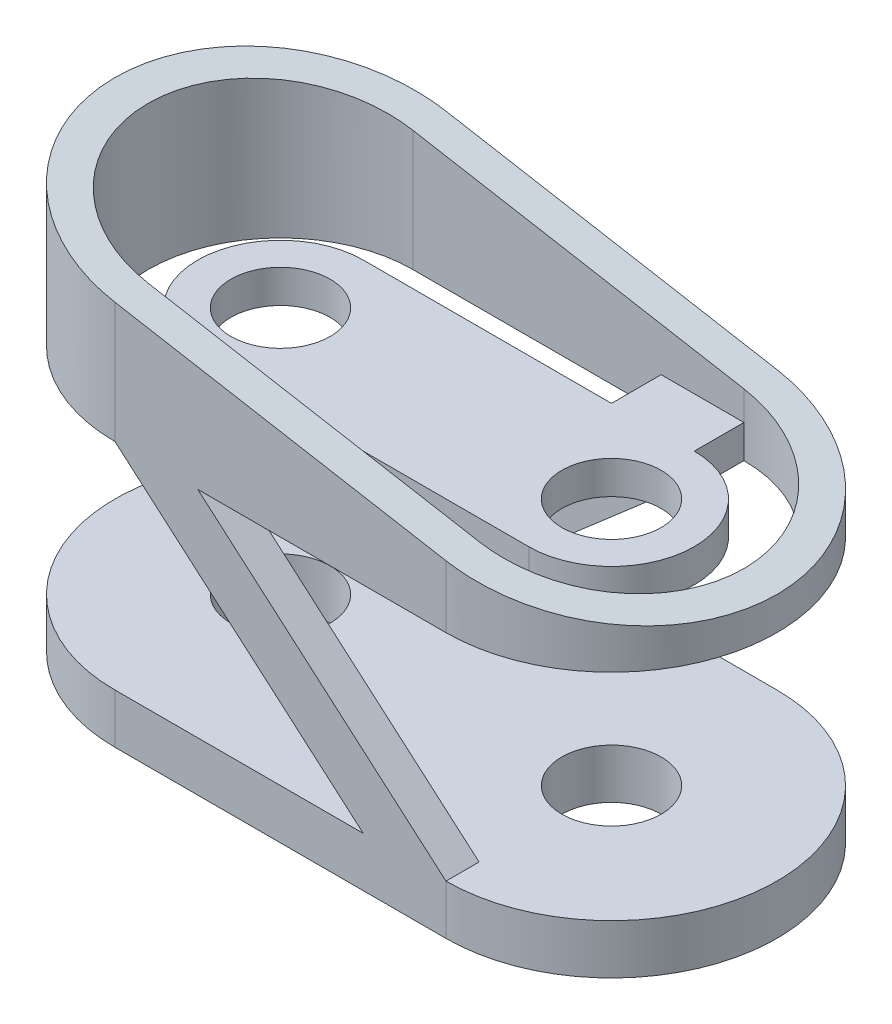
ISO-10303-21;
HEADER;
FILE_DESCRIPTION(('STEP AP214'),'2;1');
FILE_NAME('part.step','',(''),(''),'','','');
FILE_SCHEMA(('AUTOMOTIVE_DESIGN { 1 0 10303 214 1 1 1 1 }'));
ENDSEC;
DATA;
#1=APPLICATION_CONTEXT('core data for automotive mechanical design processes');
#2=APPLICATION_PROTOCOL_DEFINITION('international standard','automotive_design',2000,#1);
#3=PRODUCT_CONTEXT('',#1,'mechanical');
#4=PRODUCT('Part','Part','',(#3));
#5=PRODUCT_RELATED_PRODUCT_CATEGORY('part','',(#4));
#6=PRODUCT_DEFINITION_FORMATION('','',#4);
#7=PRODUCT_DEFINITION_CONTEXT('part definition',#1,'design');
#8=PRODUCT_DEFINITION('design','',#6,#7);
#9=PRODUCT_DEFINITION_SHAPE('','',#8);
#10=(LENGTH_UNIT() NAMED_UNIT(*) SI_UNIT(.MILLI.,.METRE.));
#11=(NAMED_UNIT(*) PLANE_ANGLE_UNIT() SI_UNIT($,.RADIAN.));
#12=(NAMED_UNIT(*) SI_UNIT($,.STERADIAN.) SOLID_ANGLE_UNIT());
#13=UNCERTAINTY_MEASURE_WITH_UNIT(LENGTH_MEASURE(1.E-05),#10,'distance_accuracy_value','');
#14=(GEOMETRIC_REPRESENTATION_CONTEXT(3) GLOBAL_UNCERTAINTY_ASSIGNED_CONTEXT((#13)) GLOBAL_UNIT_ASSIGNED_CONTEXT((#10,
#11,#12)) REPRESENTATION_CONTEXT('',''));
#15=CARTESIAN_POINT('',(0.,0.,0.));
#16=DIRECTION('',(0.,0.,1.));
#17=DIRECTION('',(1.,0.,0.));
#18=AXIS2_PLACEMENT_3D('',#15,#16,#17);
#19=CARTESIAN_POINT('',(0.,80.,0.));
#20=DIRECTION('',(0.,1.,0.));
#21=DIRECTION('',(0.,0.,1.));
#22=AXIS2_PLACEMENT_3D('',#19,#20,#21);
#23=PLANE('',#22);
#24=DIRECTION('',(-1.,0.,0.));
#25=VECTOR('',#24,1.);
#26=CARTESIAN_POINT('',(100.,80.,-50.));
#27=LINE('',#26,#25);
#28=CARTESIAN_POINT('',(75.,80.,-50.));
#29=VERTEX_POINT('',#28);
#30=CARTESIAN_POINT('',(0.,80.,-50.));
#31=VERTEX_POINT('',#30);
#32=EDGE_CURVE('E364',#29,#31,#27,.T.);
#33=ORIENTED_EDGE('',*,*,#32,.F.);
#34=DIRECTION('',(0.,0.,-1.));
#35=VECTOR('',#34,1.);
#36=CARTESIAN_POINT('',(75.,80.,-40.));
#37=LINE('',#36,#35);
#38=CARTESIAN_POINT('',(75.,80.,-40.));
#39=VERTEX_POINT('',#38);
#40=EDGE_CURVE('E470',#39,#29,#37,.T.);
#41=ORIENTED_EDGE('',*,*,#40,.F.);
#42=DIRECTION('',(-1.,0.,0.));
#43=VECTOR('',#42,1.);
#44=CARTESIAN_POINT('',(0.,80.,-40.));
#45=LINE('',#44,#43);
#46=CARTESIAN_POINT('',(0.,80.,-40.));
#47=VERTEX_POINT('',#46);
#48=EDGE_CURVE('E264',#39,#47,#45,.T.);
#49=ORIENTED_EDGE('',*,*,#48,.T.);
#50=CARTESIAN_POINT('',(0.,80.,0.));
#51=DIRECTION('',(0.,1.,0.));
#52=DIRECTION('',(0.,0.,1.));
#53=AXIS2_PLACEMENT_3D('',#50,#51,#52);
#54=CIRCLE('',#53,40.);
#55=CARTESIAN_POINT('',(0.,80.,40.));
#56=VERTEX_POINT('',#55);
#57=EDGE_CURVE('E345',#47,#56,#54,.T.);
#58=ORIENTED_EDGE('',*,*,#57,.T.);
#59=DIRECTION('',(0.,0.,1.));
#60=VECTOR('',#59,1.);
#61=CARTESIAN_POINT('',(0.,80.,40.));
#62=LINE('',#61,#60);
#63=CARTESIAN_POINT('',(0.,80.,50.));
#64=VERTEX_POINT('',#63);
#65=EDGE_CURVE('E393',#56,#64,#62,.T.);
#66=ORIENTED_EDGE('',*,*,#65,.T.);
#67=CARTESIAN_POINT('',(0.,80.,0.));
#68=DIRECTION('',(0.,1.,0.));
#69=DIRECTION('',(0.,0.,1.));
#70=AXIS2_PLACEMENT_3D('',#67,#68,#69);
#71=CIRCLE('',#70,50.);
#72=EDGE_CURVE('E358',#31,#64,#71,.T.);
#73=ORIENTED_EDGE('',*,*,#72,.F.);
#74=EDGE_LOOP('',(#33,#41,#49,#58,#66,#73));
#75=FACE_BOUND('',#74,.T.);
#76=ADVANCED_FACE('F43',(#75),#23,.F.);
#77=CARTESIAN_POINT('',(100.,80.,0.));
#78=DIRECTION('',(0.,1.,0.));
#79=DIRECTION('',(0.,0.,1.));
#80=AXIS2_PLACEMENT_3D('',#77,#78,#79);
#81=CIRCLE('',#80,40.);
#82=CARTESIAN_POINT('',(100.,80.,40.));
#83=VERTEX_POINT('',#82);
#84=CARTESIAN_POINT('',(100.,80.,-40.));
#85=VERTEX_POINT('',#84);
#86=EDGE_CURVE('E252',#83,#85,#81,.T.);
#87=ORIENTED_EDGE('',*,*,#86,.T.);
#88=DIRECTION('',(0.,0.,-1.));
#89=VECTOR('',#88,1.);
#90=CARTESIAN_POINT('',(100.,80.,-40.));
#91=LINE('',#90,#89);
#92=CARTESIAN_POINT('',(100.,80.,-50.));
#93=VERTEX_POINT('',#92);
#94=EDGE_CURVE('E209',#85,#93,#91,.T.);
#95=ORIENTED_EDGE('',*,*,#94,.T.);
#96=CARTESIAN_POINT('',(100.,80.,0.));
#97=DIRECTION('',(0.,1.,0.));
#98=DIRECTION('',(0.,0.,1.));
#99=AXIS2_PLACEMENT_3D('',#96,#97,#98);
#100=CIRCLE('',#99,50.);
#101=CARTESIAN_POINT('',(100.,80.,50.));
#102=VERTEX_POINT('',#101);
#103=EDGE_CURVE('E363',#102,#93,#100,.T.);
#104=ORIENTED_EDGE('',*,*,#103,.F.);
#105=DIRECTION('',(1.,0.,0.));
#106=VECTOR('',#105,1.);
#107=CARTESIAN_POINT('',(0.,80.,50.));
#108=LINE('',#107,#106);
#109=CARTESIAN_POINT('',(25.,80.,50.));
#110=VERTEX_POINT('',#109);
#111=EDGE_CURVE('E360',#110,#102,#108,.T.);
#112=ORIENTED_EDGE('',*,*,#111,.F.);
#113=DIRECTION('',(0.,0.,1.));
#114=VECTOR('',#113,1.);
#115=CARTESIAN_POINT('',(25.,80.,40.));
#116=LINE('',#115,#114);
#117=CARTESIAN_POINT('',(25.,80.,40.));
#118=VERTEX_POINT('',#117);
#119=EDGE_CURVE('E399',#118,#110,#116,.T.);
#120=ORIENTED_EDGE('',*,*,#119,.F.);
#121=DIRECTION('',(1.,0.,0.));
#122=VECTOR('',#121,1.);
#123=CARTESIAN_POINT('',(0.,80.,40.));
#124=LINE('',#123,#122);
#125=EDGE_CURVE('E263',#118,#83,#124,.T.);
#126=ORIENTED_EDGE('',*,*,#125,.T.);
#127=EDGE_LOOP('',(#87,#95,#104,#112,#120,#126));
#128=FACE_BOUND('',#127,.T.);
#129=ADVANCED_FACE('F258',(#128),#23,.F.);
#130=CARTESIAN_POINT('',(0.,15.,0.));
#131=DIRECTION('',(0.,-1.,0.));
#132=DIRECTION('',(0.,0.,-1.));
#133=AXIS2_PLACEMENT_3D('',#130,#131,#132);
#134=CYLINDRICAL_SURFACE('',#133,50.);
#135=CARTESIAN_POINT('',(0.,0.,0.));
#136=DIRECTION('',(0.,1.,0.));
#137=DIRECTION('',(0.,0.,1.));
#138=AXIS2_PLACEMENT_3D('',#135,#136,#137);
#139=CIRCLE('',#138,50.);
#140=CARTESIAN_POINT('',(0.,0.,-50.));
#141=VERTEX_POINT('',#140);
#142=CARTESIAN_POINT('',(0.,0.,50.));
#143=VERTEX_POINT('',#142);
#144=EDGE_CURVE('E411',#141,#143,#139,.T.);
#145=ORIENTED_EDGE('',*,*,#144,.T.);
#146=DIRECTION('',(0.,-1.,0.));
#147=VECTOR('',#146,1.);
#148=CARTESIAN_POINT('',(0.,15.,50.));
#149=LINE('',#148,#147);
#150=CARTESIAN_POINT('',(0.,15.,50.));
#151=VERTEX_POINT('',#150);
#152=EDGE_CURVE('E11',#151,#143,#149,.T.);
#153=ORIENTED_EDGE('',*,*,#152,.F.);
#154=CARTESIAN_POINT('',(0.,15.,0.));
#155=DIRECTION('',(0.,1.,0.));
#156=DIRECTION('',(0.,0.,1.));
#157=AXIS2_PLACEMENT_3D('',#154,#155,#156);
#158=CIRCLE('',#157,50.);
#159=CARTESIAN_POINT('',(0.,15.,-50.));
#160=VERTEX_POINT('',#159);
#161=EDGE_CURVE('E420',#160,#151,#158,.T.);
#162=ORIENTED_EDGE('',*,*,#161,.F.);
#163=DIRECTION('',(0.,-1.,0.));
#164=VECTOR('',#163,1.);
#165=CARTESIAN_POINT('',(0.,15.,-50.));
#166=LINE('',#165,#164);
#167=EDGE_CURVE('E431',#160,#141,#166,.T.);
#168=ORIENTED_EDGE('',*,*,#167,.T.);
#169=EDGE_LOOP('',(#145,#153,#162,#168));
#170=FACE_BOUND('',#169,.T.);
#171=ADVANCED_FACE('F44',(#170),#134,.T.);
#172=CARTESIAN_POINT('',(0.,15.,50.));
#173=DIRECTION('',(0.,0.,-1.));
#174=DIRECTION('',(-1.,0.,0.));
#175=AXIS2_PLACEMENT_3D('',#172,#173,#174);
#176=PLANE('',#175);
#177=DIRECTION('',(1.,0.,0.));
#178=VECTOR('',#177,1.);
#179=CARTESIAN_POINT('',(0.,0.,50.));
#180=LINE('',#179,#178);
#181=CARTESIAN_POINT('',(100.,0.,50.));
#182=VERTEX_POINT('',#181);
#183=EDGE_CURVE('E432',#143,#182,#180,.T.);
#184=ORIENTED_EDGE('',*,*,#183,.T.);
#185=DIRECTION('',(0.,-1.,0.));
#186=VECTOR('',#185,1.);
#187=CARTESIAN_POINT('',(100.,15.,50.));
#188=LINE('',#187,#186);
#189=CARTESIAN_POINT('',(100.,15.,50.));
#190=VERTEX_POINT('',#189);
#191=EDGE_CURVE('E51',#190,#182,#188,.T.);
#192=ORIENTED_EDGE('',*,*,#191,.F.);
#193=DIRECTION('',(-0.755689082789818,0.654930538417842,0.));
#194=VECTOR('',#193,1.);
#195=CARTESIAN_POINT('',(25.,80.,50.));
#196=LINE('',#195,#194);
#197=EDGE_CURVE('E381',#190,#110,#196,.T.);
#198=ORIENTED_EDGE('',*,*,#197,.T.);
#199=ORIENTED_EDGE('',*,*,#111,.T.);
#200=DIRECTION('',(0.,-1.,0.));
#201=VECTOR('',#200,1.);
#202=CARTESIAN_POINT('',(100.,130.,50.));
#203=LINE('',#202,#201);
#204=CARTESIAN_POINT('',(100.,98.8163490354229,50.));
#205=VERTEX_POINT('',#204);
#206=EDGE_CURVE('E371',#205,#102,#203,.T.);
#207=ORIENTED_EDGE('',*,*,#206,.F.);
#208=DIRECTION('',(0.984807753012209,-0.173648177666924,0.));
#209=VECTOR('',#208,1.);
#210=CARTESIAN_POINT('',(150.,90.,50.));
#211=LINE('',#210,#209);
#212=CARTESIAN_POINT('',(0.,116.449047106269,50.));
#213=VERTEX_POINT('',#212);
#214=EDGE_CURVE('E315',#213,#205,#211,.T.);
#215=ORIENTED_EDGE('',*,*,#214,.F.);
#216=DIRECTION('',(0.,-1.,0.));
#217=VECTOR('',#216,1.);
#218=CARTESIAN_POINT('',(0.,130.,50.));
#219=LINE('',#218,#217);
#220=EDGE_CURVE('E372',#213,#64,#219,.T.);
#221=ORIENTED_EDGE('',*,*,#220,.T.);
#222=DIRECTION('',(0.755689082789818,-0.654930538417842,0.));
#223=VECTOR('',#222,1.);
#224=CARTESIAN_POINT('',(0.,80.,50.));
#225=LINE('',#224,#223);
#226=CARTESIAN_POINT('',(75.,15.,50.));
#227=VERTEX_POINT('',#226);
#228=EDGE_CURVE('E378',#64,#227,#225,.T.);
#229=ORIENTED_EDGE('',*,*,#228,.T.);
#230=DIRECTION('',(1.,0.,0.));
#231=VECTOR('',#230,1.);
#232=CARTESIAN_POINT('',(0.,15.,50.));
#233=LINE('',#232,#231);
#234=EDGE_CURVE('E421',#151,#227,#233,.T.);
#235=ORIENTED_EDGE('',*,*,#234,.F.);
#236=ORIENTED_EDGE('',*,*,#152,.T.);
#237=EDGE_LOOP('',(#184,#192,#198,#199,#207,#215,#221,#229,#235,#236));
#238=FACE_BOUND('',#237,.T.);
#239=ADVANCED_FACE('F581',(#238),#176,.F.);
#240=CARTESIAN_POINT('',(100.,15.,0.));
#241=DIRECTION('',(0.,-1.,0.));
#242=DIRECTION('',(0.,0.,-1.));
#243=AXIS2_PLACEMENT_3D('',#240,#241,#242);
#244=CYLINDRICAL_SURFACE('',#243,50.);
#245=CARTESIAN_POINT('',(100.,0.,0.));
#246=DIRECTION('',(0.,1.,0.));
#247=DIRECTION('',(0.,0.,1.));
#248=AXIS2_PLACEMENT_3D('',#245,#246,#247);
#249=CIRCLE('',#248,50.);
#250=CARTESIAN_POINT('',(100.,0.,-50.));
#251=VERTEX_POINT('',#250);
#252=EDGE_CURVE('E436',#182,#251,#249,.T.);
#253=ORIENTED_EDGE('',*,*,#252,.T.);
#254=DIRECTION('',(0.,-1.,0.));
#255=VECTOR('',#254,1.);
#256=CARTESIAN_POINT('',(100.,15.,-50.));
#257=LINE('',#256,#255);
#258=CARTESIAN_POINT('',(100.,15.,-50.));
#259=VERTEX_POINT('',#258);
#260=EDGE_CURVE('E441',#259,#251,#257,.T.);
#261=ORIENTED_EDGE('',*,*,#260,.F.);
#262=CARTESIAN_POINT('',(100.,15.,0.));
#263=DIRECTION('',(0.,1.,0.));
#264=DIRECTION('',(0.,0.,1.));
#265=AXIS2_PLACEMENT_3D('',#262,#263,#264);
#266=CIRCLE('',#265,50.);
#267=EDGE_CURVE('E430',#190,#259,#266,.T.);
#268=ORIENTED_EDGE('',*,*,#267,.F.);
#269=ORIENTED_EDGE('',*,*,#191,.T.);
#270=EDGE_LOOP('',(#253,#261,#268,#269));
#271=FACE_BOUND('',#270,.T.);
#272=ADVANCED_FACE('F449',(#271),#244,.T.);
#273=CARTESIAN_POINT('',(0.,15.,-50.));
#274=DIRECTION('',(0.,0.,1.));
#275=DIRECTION('',(1.,0.,0.));
#276=AXIS2_PLACEMENT_3D('',#273,#274,#275);
#277=PLANE('',#276);
#278=DIRECTION('',(-1.,0.,0.));
#279=VECTOR('',#278,1.);
#280=CARTESIAN_POINT('',(0.,0.,-50.));
#281=LINE('',#280,#279);
#282=EDGE_CURVE('E425',#251,#141,#281,.T.);
#283=ORIENTED_EDGE('',*,*,#282,.T.);
#284=ORIENTED_EDGE('',*,*,#167,.F.);
#285=DIRECTION('',(0.755689082789818,0.654930538417842,0.));
#286=VECTOR('',#285,1.);
#287=CARTESIAN_POINT('',(75.,80.,-50.));
#288=LINE('',#287,#286);
#289=EDGE_CURVE('E241',#160,#29,#288,.T.);
#290=ORIENTED_EDGE('',*,*,#289,.T.);
#291=ORIENTED_EDGE('',*,*,#32,.T.);
#292=DIRECTION('',(0.,-1.,0.));
#293=VECTOR('',#292,1.);
#294=CARTESIAN_POINT('',(0.,130.,-50.));
#295=LINE('',#294,#293);
#296=CARTESIAN_POINT('',(0.,116.449047106269,-50.));
#297=VERTEX_POINT('',#296);
#298=EDGE_CURVE('E366',#297,#31,#295,.T.);
#299=ORIENTED_EDGE('',*,*,#298,.F.);
#300=DIRECTION('',(0.984807753012209,-0.173648177666924,0.));
#301=VECTOR('',#300,1.);
#302=CARTESIAN_POINT('',(150.,90.,-50.));
#303=LINE('',#302,#301);
#304=CARTESIAN_POINT('',(100.,98.8163490354229,-50.));
#305=VERTEX_POINT('',#304);
#306=EDGE_CURVE('E330',#297,#305,#303,.T.);
#307=ORIENTED_EDGE('',*,*,#306,.T.);
#308=DIRECTION('',(0.,-1.,0.));
#309=VECTOR('',#308,1.);
#310=CARTESIAN_POINT('',(100.,130.,-50.));
#311=LINE('',#310,#309);
#312=EDGE_CURVE('E367',#305,#93,#311,.T.);
#313=ORIENTED_EDGE('',*,*,#312,.T.);
#314=DIRECTION('',(-0.755689082789818,-0.654930538417842,0.));
#315=VECTOR('',#314,1.);
#316=CARTESIAN_POINT('',(100.,80.,-50.));
#317=LINE('',#316,#315);
#318=CARTESIAN_POINT('',(25.,15.,-50.));
#319=VERTEX_POINT('',#318);
#320=EDGE_CURVE('E211',#93,#319,#317,.T.);
#321=ORIENTED_EDGE('',*,*,#320,.T.);
#322=DIRECTION('',(-1.,0.,0.));
#323=VECTOR('',#322,1.);
#324=CARTESIAN_POINT('',(0.,15.,-50.));
#325=LINE('',#324,#323);
#326=EDGE_CURVE('E429',#259,#319,#325,.T.);
#327=ORIENTED_EDGE('',*,*,#326,.F.);
#328=ORIENTED_EDGE('',*,*,#260,.T.);
#329=EDGE_LOOP('',(#283,#284,#290,#291,#299,#307,#313,#321,#327,#328));
#330=FACE_BOUND('',#329,.T.);
#331=ADVANCED_FACE('F460',(#330),#277,.F.);
#332=CARTESIAN_POINT('',(0.,15.,0.));
#333=DIRECTION('',(0.,1.,0.));
#334=DIRECTION('',(0.,0.,1.));
#335=AXIS2_PLACEMENT_3D('',#332,#333,#334);
#336=PLANE('',#335);
#337=DIRECTION('',(0.,0.,-1.));
#338=VECTOR('',#337,1.);
#339=CARTESIAN_POINT('',(0.,15.,-40.));
#340=LINE('',#339,#338);
#341=CARTESIAN_POINT('',(0.,15.,-40.));
#342=VERTEX_POINT('',#341);
#343=EDGE_CURVE('E463',#342,#160,#340,.T.);
#344=ORIENTED_EDGE('',*,*,#343,.T.);
#345=ORIENTED_EDGE('',*,*,#161,.T.);
#346=ORIENTED_EDGE('',*,*,#234,.T.);
#347=DIRECTION('',(0.,0.,1.));
#348=VECTOR('',#347,1.);
#349=CARTESIAN_POINT('',(75.,15.,40.));
#350=LINE('',#349,#348);
#351=CARTESIAN_POINT('',(75.,15.,40.));
#352=VERTEX_POINT('',#351);
#353=EDGE_CURVE('E404',#352,#227,#350,.T.);
#354=ORIENTED_EDGE('',*,*,#353,.F.);
#355=DIRECTION('',(1.,0.,0.));
#356=VECTOR('',#355,1.);
#357=CARTESIAN_POINT('',(75.,15.,40.));
#358=LINE('',#357,#356);
#359=CARTESIAN_POINT('',(100.,15.,40.));
#360=VERTEX_POINT('',#359);
#361=EDGE_CURVE('E390',#352,#360,#358,.T.);
#362=ORIENTED_EDGE('',*,*,#361,.T.);
#363=DIRECTION('',(0.,0.,1.));
#364=VECTOR('',#363,1.);
#365=CARTESIAN_POINT('',(100.,15.,40.));
#366=LINE('',#365,#364);
#367=EDGE_CURVE('E402',#360,#190,#366,.T.);
#368=ORIENTED_EDGE('',*,*,#367,.T.);
#369=ORIENTED_EDGE('',*,*,#267,.T.);
#370=ORIENTED_EDGE('',*,*,#326,.T.);
#371=DIRECTION('',(0.,0.,-1.));
#372=VECTOR('',#371,1.);
#373=CARTESIAN_POINT('',(25.,15.,-40.));
#374=LINE('',#373,#372);
#375=CARTESIAN_POINT('',(25.,15.,-40.));
#376=VERTEX_POINT('',#375);
#377=EDGE_CURVE('E59',#376,#319,#374,.T.);
#378=ORIENTED_EDGE('',*,*,#377,.F.);
#379=DIRECTION('',(-1.,0.,0.));
#380=VECTOR('',#379,1.);
#381=CARTESIAN_POINT('',(25.,15.,-40.));
#382=LINE('',#381,#380);
#383=EDGE_CURVE('E65',#376,#342,#382,.T.);
#384=ORIENTED_EDGE('',*,*,#383,.T.);
#385=EDGE_LOOP('',(#344,#345,#346,#354,#362,#368,#369,#370,#378,#384));
#386=FACE_BOUND('',#385,.T.);
#387=CARTESIAN_POINT('',(100.,15.,0.));
#388=DIRECTION('',(0.,1.,0.));
#389=DIRECTION('',(0.,0.,1.));
#390=AXIS2_PLACEMENT_3D('',#387,#388,#389);
#391=CIRCLE('',#390,15.);
#392=CARTESIAN_POINT('',(100.,15.,15.));
#393=VERTEX_POINT('',#392);
#394=EDGE_CURVE('E415',#393,#393,#391,.T.);
#395=ORIENTED_EDGE('',*,*,#394,.F.);
#396=EDGE_LOOP('',(#395));
#397=FACE_BOUND('',#396,.T.);
#398=CARTESIAN_POINT('',(0.,15.,0.));
#399=DIRECTION('',(0.,1.,0.));
#400=DIRECTION('',(0.,0.,1.));
#401=AXIS2_PLACEMENT_3D('',#398,#399,#400);
#402=CIRCLE('',#401,15.);
#403=CARTESIAN_POINT('',(0.,15.,15.));
#404=VERTEX_POINT('',#403);
#405=EDGE_CURVE('E400',#404,#404,#402,.T.);
#406=ORIENTED_EDGE('',*,*,#405,.F.);
#407=EDGE_LOOP('',(#406));
#408=FACE_BOUND('',#407,.T.);
#409=ADVANCED_FACE('F461',(#386,#397,#408),#336,.T.);
#410=CARTESIAN_POINT('',(0.,0.,0.));
#411=DIRECTION('',(0.,1.,0.));
#412=DIRECTION('',(0.,0.,1.));
#413=AXIS2_PLACEMENT_3D('',#410,#411,#412);
#414=PLANE('',#413);
#415=CARTESIAN_POINT('',(100.,0.,0.));
#416=DIRECTION('',(0.,1.,0.));
#417=DIRECTION('',(0.,0.,1.));
#418=AXIS2_PLACEMENT_3D('',#415,#416,#417);
#419=CIRCLE('',#418,15.);
#420=CARTESIAN_POINT('',(100.,0.,15.));
#421=VERTEX_POINT('',#420);
#422=EDGE_CURVE('E409',#421,#421,#419,.T.);
#423=ORIENTED_EDGE('',*,*,#422,.T.);
#424=EDGE_LOOP('',(#423));
#425=FACE_BOUND('',#424,.T.);
#426=CARTESIAN_POINT('',(0.,0.,0.));
#427=DIRECTION('',(0.,1.,0.));
#428=DIRECTION('',(0.,0.,1.));
#429=AXIS2_PLACEMENT_3D('',#426,#427,#428);
#430=CIRCLE('',#429,15.);
#431=CARTESIAN_POINT('',(0.,0.,15.));
#432=VERTEX_POINT('',#431);
#433=EDGE_CURVE('E414',#432,#432,#430,.T.);
#434=ORIENTED_EDGE('',*,*,#433,.T.);
#435=EDGE_LOOP('',(#434));
#436=FACE_BOUND('',#435,.T.);
#437=ORIENTED_EDGE('',*,*,#144,.F.);
#438=ORIENTED_EDGE('',*,*,#282,.F.);
#439=ORIENTED_EDGE('',*,*,#252,.F.);
#440=ORIENTED_EDGE('',*,*,#183,.F.);
#441=EDGE_LOOP('',(#437,#438,#439,#440));
#442=FACE_BOUND('',#441,.T.);
#443=ADVANCED_FACE('F451',(#425,#436,#442),#414,.F.);
#444=CARTESIAN_POINT('',(0.,0.,0.));
#445=DIRECTION('',(0.,1.,0.));
#446=DIRECTION('',(0.,0.,1.));
#447=AXIS2_PLACEMENT_3D('',#444,#445,#446);
#448=CYLINDRICAL_SURFACE('',#447,15.);
#449=ORIENTED_EDGE('',*,*,#433,.F.);
#450=EDGE_LOOP('',(#449));
#451=FACE_BOUND('',#450,.T.);
#452=ORIENTED_EDGE('',*,*,#405,.T.);
#453=EDGE_LOOP('',(#452));
#454=FACE_BOUND('',#453,.T.);
#455=ADVANCED_FACE('F575',(#451,#454),#448,.F.);
#456=CARTESIAN_POINT('',(100.,0.,0.));
#457=DIRECTION('',(0.,1.,0.));
#458=DIRECTION('',(0.,0.,1.));
#459=AXIS2_PLACEMENT_3D('',#456,#457,#458);
#460=CYLINDRICAL_SURFACE('',#459,15.);
#461=ORIENTED_EDGE('',*,*,#422,.F.);
#462=EDGE_LOOP('',(#461));
#463=FACE_BOUND('',#462,.T.);
#464=ORIENTED_EDGE('',*,*,#394,.T.);
#465=EDGE_LOOP('',(#464));
#466=FACE_BOUND('',#465,.T.);
#467=ADVANCED_FACE('F570',(#463,#466),#460,.F.);
#468=CARTESIAN_POINT('',(25.,80.,40.));
#469=DIRECTION('',(0.654930538417842,0.755689082789818,0.));
#470=DIRECTION('',(-0.755689082789818,0.654930538417842,0.));
#471=AXIS2_PLACEMENT_3D('',#468,#469,#470);
#472=PLANE('',#471);
#473=ORIENTED_EDGE('',*,*,#197,.F.);
#474=ORIENTED_EDGE('',*,*,#367,.F.);
#475=DIRECTION('',(-0.755689082789818,0.654930538417842,0.));
#476=VECTOR('',#475,1.);
#477=CARTESIAN_POINT('',(25.,80.,40.));
#478=LINE('',#477,#476);
#479=EDGE_CURVE('E388',#360,#118,#478,.T.);
#480=ORIENTED_EDGE('',*,*,#479,.T.);
#481=ORIENTED_EDGE('',*,*,#119,.T.);
#482=EDGE_LOOP('',(#473,#474,#480,#481));
#483=FACE_BOUND('',#482,.T.);
#484=ADVANCED_FACE('F565',(#483),#472,.T.);
#485=CARTESIAN_POINT('',(0.,80.,40.));
#486=DIRECTION('',(-0.654930538417842,-0.755689082789818,0.));
#487=DIRECTION('',(0.755689082789818,-0.654930538417842,0.));
#488=AXIS2_PLACEMENT_3D('',#485,#486,#487);
#489=PLANE('',#488);
#490=ORIENTED_EDGE('',*,*,#228,.F.);
#491=ORIENTED_EDGE('',*,*,#65,.F.);
#492=DIRECTION('',(0.755689082789818,-0.654930538417842,0.));
#493=VECTOR('',#492,1.);
#494=CARTESIAN_POINT('',(0.,80.,40.));
#495=LINE('',#494,#493);
#496=EDGE_CURVE('E384',#56,#352,#495,.T.);
#497=ORIENTED_EDGE('',*,*,#496,.T.);
#498=ORIENTED_EDGE('',*,*,#353,.T.);
#499=EDGE_LOOP('',(#490,#491,#497,#498));
#500=FACE_BOUND('',#499,.T.);
#501=ADVANCED_FACE('F558',(#500),#489,.T.);
#502=CARTESIAN_POINT('',(0.,0.,40.));
#503=DIRECTION('',(0.,0.,-1.));
#504=DIRECTION('',(-1.,0.,0.));
#505=AXIS2_PLACEMENT_3D('',#502,#503,#504);
#506=PLANE('',#505);
#507=DIRECTION('',(-1.,0.,0.));
#508=VECTOR('',#507,1.);
#509=CARTESIAN_POINT('',(0.,80.,40.));
#510=LINE('',#509,#508);
#511=EDGE_CURVE('E379',#118,#56,#510,.T.);
#512=ORIENTED_EDGE('',*,*,#511,.F.);
#513=ORIENTED_EDGE('',*,*,#479,.F.);
#514=ORIENTED_EDGE('',*,*,#361,.F.);
#515=ORIENTED_EDGE('',*,*,#496,.F.);
#516=EDGE_LOOP('',(#512,#513,#514,#515));
#517=FACE_BOUND('',#516,.T.);
#518=ADVANCED_FACE('F546',(#517),#506,.T.);
#519=DIRECTION('',(0.,0.,1.));
#520=VECTOR('',#519,1.);
#521=CARTESIAN_POINT('',(75.,80.,-25.));
#522=LINE('',#521,#520);
#523=CARTESIAN_POINT('',(75.,80.,-25.));
#524=VERTEX_POINT('',#523);
#525=EDGE_CURVE('E239',#39,#524,#522,.T.);
#526=ORIENTED_EDGE('',*,*,#525,.F.);
#527=DIRECTION('',(1.,0.,0.));
#528=VECTOR('',#527,1.);
#529=CARTESIAN_POINT('',(100.,80.,-40.));
#530=LINE('',#529,#528);
#531=EDGE_CURVE('E225',#39,#85,#530,.T.);
#532=ORIENTED_EDGE('',*,*,#531,.T.);
#533=DIRECTION('',(0.,0.,-1.));
#534=VECTOR('',#533,1.);
#535=CARTESIAN_POINT('',(100.,80.,-25.));
#536=LINE('',#535,#534);
#537=CARTESIAN_POINT('',(100.,80.,-25.));
#538=VERTEX_POINT('',#537);
#539=EDGE_CURVE('E236',#538,#85,#536,.T.);
#540=ORIENTED_EDGE('',*,*,#539,.F.);
#541=CARTESIAN_POINT('',(100.,80.,0.));
#542=DIRECTION('',(0.,1.,0.));
#543=DIRECTION('',(0.,0.,1.));
#544=AXIS2_PLACEMENT_3D('',#541,#542,#543);
#545=CIRCLE('',#544,25.);
#546=CARTESIAN_POINT('',(100.,80.,25.));
#547=VERTEX_POINT('',#546);
#548=EDGE_CURVE('E269',#547,#538,#545,.T.);
#549=ORIENTED_EDGE('',*,*,#548,.F.);
#550=DIRECTION('',(1.,0.,0.));
#551=VECTOR('',#550,1.);
#552=CARTESIAN_POINT('',(25.,80.,25.));
#553=LINE('',#552,#551);
#554=CARTESIAN_POINT('',(25.,80.,25.));
#555=VERTEX_POINT('',#554);
#556=EDGE_CURVE('E275',#555,#547,#553,.T.);
#557=ORIENTED_EDGE('',*,*,#556,.F.);
#558=DIRECTION('',(0.,0.,-1.));
#559=VECTOR('',#558,1.);
#560=CARTESIAN_POINT('',(25.,80.,25.));
#561=LINE('',#560,#559);
#562=EDGE_CURVE('E492',#118,#555,#561,.T.);
#563=ORIENTED_EDGE('',*,*,#562,.F.);
#564=ORIENTED_EDGE('',*,*,#511,.T.);
#565=DIRECTION('',(0.,0.,1.));
#566=VECTOR('',#565,1.);
#567=CARTESIAN_POINT('',(0.,80.,25.));
#568=LINE('',#567,#566);
#569=CARTESIAN_POINT('',(0.,80.,25.));
#570=VERTEX_POINT('',#569);
#571=EDGE_CURVE('E495',#570,#56,#568,.T.);
#572=ORIENTED_EDGE('',*,*,#571,.F.);
#573=CARTESIAN_POINT('',(0.,80.,0.));
#574=DIRECTION('',(0.,1.,0.));
#575=DIRECTION('',(0.,0.,1.));
#576=AXIS2_PLACEMENT_3D('',#573,#574,#575);
#577=CIRCLE('',#576,25.);
#578=CARTESIAN_POINT('',(0.,80.,-25.));
#579=VERTEX_POINT('',#578);
#580=EDGE_CURVE('E307',#579,#570,#577,.T.);
#581=ORIENTED_EDGE('',*,*,#580,.F.);
#582=DIRECTION('',(-1.,0.,0.));
#583=VECTOR('',#582,1.);
#584=CARTESIAN_POINT('',(0.,80.,-25.));
#585=LINE('',#584,#583);
#586=EDGE_CURVE('E270',#524,#579,#585,.T.);
#587=ORIENTED_EDGE('',*,*,#586,.F.);
#588=EDGE_LOOP('',(#526,#532,#540,#549,#557,#563,#564,#572,#581,#587));
#589=FACE_BOUND('',#588,.T.);
#590=CARTESIAN_POINT('',(100.,80.,0.));
#591=DIRECTION('',(0.,1.,0.));
#592=DIRECTION('',(0.,0.,1.));
#593=AXIS2_PLACEMENT_3D('',#590,#591,#592);
#594=CIRCLE('',#593,15.);
#595=CARTESIAN_POINT('',(100.,80.,15.));
#596=VERTEX_POINT('',#595);
#597=EDGE_CURVE('E283',#596,#596,#594,.T.);
#598=ORIENTED_EDGE('',*,*,#597,.T.);
#599=EDGE_LOOP('',(#598));
#600=FACE_BOUND('',#599,.T.);
#601=CARTESIAN_POINT('',(0.,80.,0.));
#602=DIRECTION('',(0.,1.,0.));
#603=DIRECTION('',(0.,0.,1.));
#604=AXIS2_PLACEMENT_3D('',#601,#602,#603);
#605=CIRCLE('',#604,15.);
#606=CARTESIAN_POINT('',(0.,80.,15.));
#607=VERTEX_POINT('',#606);
#608=EDGE_CURVE('E485',#607,#607,#605,.T.);
#609=ORIENTED_EDGE('',*,*,#608,.T.);
#610=EDGE_LOOP('',(#609));
#611=FACE_BOUND('',#610,.T.);
#612=ADVANCED_FACE('F235',(#589,#600,#611),#23,.F.);
#613=CARTESIAN_POINT('',(0.,130.,0.));
#614=DIRECTION('',(0.,-1.,0.));
#615=DIRECTION('',(0.,0.,-1.));
#616=AXIS2_PLACEMENT_3D('',#613,#614,#615);
#617=CYLINDRICAL_SURFACE('',#616,50.);
#618=ORIENTED_EDGE('',*,*,#220,.F.);
#619=CARTESIAN_POINT('',(0.,116.449047106269,0.));
#620=DIRECTION('',(-0.173648177666924,-0.984807753012209,0.));
#621=DIRECTION('',(0.984807753012209,-0.173648177666924,0.));
#622=AXIS2_PLACEMENT_3D('',#619,#620,#621);
#623=ELLIPSE('',#622,50.7713305942872,50.);
#624=EDGE_CURVE('E338',#213,#297,#623,.T.);
#625=ORIENTED_EDGE('',*,*,#624,.T.);
#626=ORIENTED_EDGE('',*,*,#298,.T.);
#627=ORIENTED_EDGE('',*,*,#72,.T.);
#628=EDGE_LOOP('',(#618,#625,#626,#627));
#629=FACE_BOUND('',#628,.T.);
#630=ADVANCED_FACE('F544',(#629),#617,.T.);
#631=CARTESIAN_POINT('',(100.,130.,0.));
#632=DIRECTION('',(0.,-1.,0.));
#633=DIRECTION('',(0.,0.,-1.));
#634=AXIS2_PLACEMENT_3D('',#631,#632,#633);
#635=CYLINDRICAL_SURFACE('',#634,50.);
#636=CARTESIAN_POINT('',(100.,98.8163490354229,0.));
#637=DIRECTION('',(-0.173648177666924,-0.984807753012209,0.));
#638=DIRECTION('',(0.984807753012209,-0.173648177666924,0.));
#639=AXIS2_PLACEMENT_3D('',#636,#637,#638);
#640=ELLIPSE('',#639,50.7713305942872,50.);
#641=EDGE_CURVE('E336',#305,#205,#640,.T.);
#642=ORIENTED_EDGE('',*,*,#641,.T.);
#643=ORIENTED_EDGE('',*,*,#206,.T.);
#644=ORIENTED_EDGE('',*,*,#103,.T.);
#645=ORIENTED_EDGE('',*,*,#312,.F.);
#646=EDGE_LOOP('',(#642,#643,#644,#645));
#647=FACE_BOUND('',#646,.T.);
#648=ADVANCED_FACE('F552',(#647),#635,.T.);
#649=CARTESIAN_POINT('',(0.,130.,0.));
#650=DIRECTION('',(0.,-1.,0.));
#651=DIRECTION('',(0.,0.,-1.));
#652=AXIS2_PLACEMENT_3D('',#649,#650,#651);
#653=CYLINDRICAL_SURFACE('',#652,40.);
#654=CARTESIAN_POINT('',(0.,116.449047106269,0.));
#655=DIRECTION('',(-0.173648177666924,-0.984807753012209,0.));
#656=DIRECTION('',(0.984807753012209,-0.173648177666924,0.));
#657=AXIS2_PLACEMENT_3D('',#654,#655,#656);
#658=ELLIPSE('',#657,40.6170644754297,40.);
#659=CARTESIAN_POINT('',(0.,116.449047106269,40.));
#660=VERTEX_POINT('',#659);
#661=CARTESIAN_POINT('',(0.,116.449047106269,-40.));
#662=VERTEX_POINT('',#661);
#663=EDGE_CURVE('E337',#660,#662,#658,.T.);
#664=ORIENTED_EDGE('',*,*,#663,.F.);
#665=DIRECTION('',(0.,-1.,0.));
#666=VECTOR('',#665,1.);
#667=CARTESIAN_POINT('',(0.,130.,40.));
#668=LINE('',#667,#666);
#669=CARTESIAN_POINT('',(0.,90.,40.));
#670=VERTEX_POINT('',#669);
#671=EDGE_CURVE('E354',#660,#670,#668,.T.);
#672=ORIENTED_EDGE('',*,*,#671,.T.);
#673=DIRECTION('',(0.,1.,0.));
#674=VECTOR('',#673,1.);
#675=CARTESIAN_POINT('',(2.61861100413235E-13,80.,40.));
#676=LINE('',#675,#674);
#677=EDGE_CURVE('E324',#56,#670,#676,.T.);
#678=ORIENTED_EDGE('',*,*,#677,.F.);
#679=ORIENTED_EDGE('',*,*,#57,.F.);
#680=DIRECTION('',(0.,-1.,0.));
#681=VECTOR('',#680,1.);
#682=CARTESIAN_POINT('',(0.,130.,-40.));
#683=LINE('',#682,#681);
#684=EDGE_CURVE('E350',#662,#47,#683,.T.);
#685=ORIENTED_EDGE('',*,*,#684,.F.);
#686=EDGE_LOOP('',(#664,#672,#678,#679,#685));
#687=FACE_BOUND('',#686,.T.);
#688=ADVANCED_FACE('F792',(#687),#653,.F.);
#689=CARTESIAN_POINT('',(0.,130.,40.));
#690=DIRECTION('',(0.,0.,-1.));
#691=DIRECTION('',(-1.,0.,0.));
#692=AXIS2_PLACEMENT_3D('',#689,#690,#691);
#693=PLANE('',#692);
#694=DIRECTION('',(0.,1.,0.));
#695=VECTOR('',#694,1.);
#696=CARTESIAN_POINT('',(25.,80.,40.));
#697=LINE('',#696,#695);
#698=CARTESIAN_POINT('',(25.,90.,40.));
#699=VERTEX_POINT('',#698);
#700=EDGE_CURVE('E322',#118,#699,#697,.T.);
#701=ORIENTED_EDGE('',*,*,#700,.T.);
#702=DIRECTION('',(1.,0.,0.));
#703=VECTOR('',#702,1.);
#704=CARTESIAN_POINT('',(2.61861100413235E-13,90.,40.));
#705=LINE('',#704,#703);
#706=EDGE_CURVE('E286',#670,#699,#705,.T.);
#707=ORIENTED_EDGE('',*,*,#706,.F.);
#708=ORIENTED_EDGE('',*,*,#671,.F.);
#709=DIRECTION('',(-0.984807753012209,0.173648177666924,0.));
#710=VECTOR('',#709,1.);
#711=CARTESIAN_POINT('',(-2.31734942545659,116.857658333706,40.));
#712=LINE('',#711,#710);
#713=CARTESIAN_POINT('',(100.,98.8163490354229,40.));
#714=VERTEX_POINT('',#713);
#715=EDGE_CURVE('E333',#714,#660,#712,.T.);
#716=ORIENTED_EDGE('',*,*,#715,.F.);
#717=DIRECTION('',(0.,-1.,0.));
#718=VECTOR('',#717,1.);
#719=CARTESIAN_POINT('',(100.,130.,40.));
#720=LINE('',#719,#718);
#721=EDGE_CURVE('E351',#714,#83,#720,.T.);
#722=ORIENTED_EDGE('',*,*,#721,.T.);
#723=ORIENTED_EDGE('',*,*,#125,.F.);
#724=EDGE_LOOP('',(#701,#707,#708,#716,#722,#723));
#725=FACE_BOUND('',#724,.T.);
#726=ADVANCED_FACE('F508',(#725),#693,.T.);
#727=CARTESIAN_POINT('',(100.,130.,0.));
#728=DIRECTION('',(0.,-1.,0.));
#729=DIRECTION('',(0.,0.,-1.));
#730=AXIS2_PLACEMENT_3D('',#727,#728,#729);
#731=CYLINDRICAL_SURFACE('',#730,40.);
#732=CARTESIAN_POINT('',(100.,98.8163490354229,0.));
#733=DIRECTION('',(-0.173648177666924,-0.984807753012209,0.));
#734=DIRECTION('',(0.984807753012209,-0.173648177666924,0.));
#735=AXIS2_PLACEMENT_3D('',#732,#733,#734);
#736=ELLIPSE('',#735,40.6170644754298,40.);
#737=CARTESIAN_POINT('',(100.,98.8163490354229,-40.));
#738=VERTEX_POINT('',#737);
#739=EDGE_CURVE('E329',#738,#714,#736,.T.);
#740=ORIENTED_EDGE('',*,*,#739,.F.);
#741=DIRECTION('',(0.,-1.,0.));
#742=VECTOR('',#741,1.);
#743=CARTESIAN_POINT('',(100.,130.,-40.));
#744=LINE('',#743,#742);
#745=CARTESIAN_POINT('',(100.,90.,-40.));
#746=VERTEX_POINT('',#745);
#747=EDGE_CURVE('E254',#738,#746,#744,.T.);
#748=ORIENTED_EDGE('',*,*,#747,.T.);
#749=DIRECTION('',(0.,1.,0.));
#750=VECTOR('',#749,1.);
#751=CARTESIAN_POINT('',(99.9999999999999,80.,-40.));
#752=LINE('',#751,#750);
#753=EDGE_CURVE('E250',#85,#746,#752,.T.);
#754=ORIENTED_EDGE('',*,*,#753,.F.);
#755=ORIENTED_EDGE('',*,*,#86,.F.);
#756=ORIENTED_EDGE('',*,*,#721,.F.);
#757=EDGE_LOOP('',(#740,#748,#754,#755,#756));
#758=FACE_BOUND('',#757,.T.);
#759=ADVANCED_FACE('F248',(#758),#731,.F.);
#760=CARTESIAN_POINT('',(0.,130.,-40.));
#761=DIRECTION('',(0.,0.,1.));
#762=DIRECTION('',(1.,0.,0.));
#763=AXIS2_PLACEMENT_3D('',#760,#761,#762);
#764=PLANE('',#763);
#765=DIRECTION('',(0.,1.,0.));
#766=VECTOR('',#765,1.);
#767=CARTESIAN_POINT('',(75.,80.,-40.));
#768=LINE('',#767,#766);
#769=CARTESIAN_POINT('',(75.,90.,-40.));
#770=VERTEX_POINT('',#769);
#771=EDGE_CURVE('E260',#39,#770,#768,.T.);
#772=ORIENTED_EDGE('',*,*,#771,.T.);
#773=DIRECTION('',(-1.,0.,0.));
#774=VECTOR('',#773,1.);
#775=CARTESIAN_POINT('',(99.9999999999999,90.,-40.));
#776=LINE('',#775,#774);
#777=EDGE_CURVE('E297',#746,#770,#776,.T.);
#778=ORIENTED_EDGE('',*,*,#777,.F.);
#779=ORIENTED_EDGE('',*,*,#747,.F.);
#780=DIRECTION('',(0.984807753012209,-0.173648177666924,0.));
#781=VECTOR('',#780,1.);
#782=CARTESIAN_POINT('',(-2.3173494254566,116.857658333706,-40.));
#783=LINE('',#782,#781);
#784=EDGE_CURVE('E380',#662,#738,#783,.T.);
#785=ORIENTED_EDGE('',*,*,#784,.F.);
#786=ORIENTED_EDGE('',*,*,#684,.T.);
#787=ORIENTED_EDGE('',*,*,#48,.F.);
#788=EDGE_LOOP('',(#772,#778,#779,#785,#786,#787));
#789=FACE_BOUND('',#788,.T.);
#790=ADVANCED_FACE('F513',(#789),#764,.T.);
#791=CARTESIAN_POINT('',(150.,90.,-50.));
#792=DIRECTION('',(-0.173648177666924,-0.984807753012209,0.));
#793=DIRECTION('',(0.984807753012209,-0.173648177666924,0.));
#794=AXIS2_PLACEMENT_3D('',#791,#792,#793);
#795=PLANE('',#794);
#796=ORIENTED_EDGE('',*,*,#663,.T.);
#797=ORIENTED_EDGE('',*,*,#784,.T.);
#798=ORIENTED_EDGE('',*,*,#739,.T.);
#799=ORIENTED_EDGE('',*,*,#715,.T.);
#800=EDGE_LOOP('',(#796,#797,#798,#799));
#801=FACE_BOUND('',#800,.T.);
#802=ORIENTED_EDGE('',*,*,#214,.T.);
#803=ORIENTED_EDGE('',*,*,#641,.F.);
#804=ORIENTED_EDGE('',*,*,#306,.F.);
#805=ORIENTED_EDGE('',*,*,#624,.F.);
#806=EDGE_LOOP('',(#802,#803,#804,#805));
#807=FACE_BOUND('',#806,.T.);
#808=ADVANCED_FACE('F825',(#801,#807),#795,.F.);
#809=CARTESIAN_POINT('',(0.,80.,0.));
#810=DIRECTION('',(0.,1.,0.));
#811=DIRECTION('',(0.,0.,1.));
#812=AXIS2_PLACEMENT_3D('',#809,#810,#811);
#813=CYLINDRICAL_SURFACE('',#812,25.);
#814=CARTESIAN_POINT('',(0.,90.,0.));
#815=DIRECTION('',(0.,1.,0.));
#816=DIRECTION('',(0.,0.,1.));
#817=AXIS2_PLACEMENT_3D('',#814,#815,#816);
#818=CIRCLE('',#817,25.);
#819=CARTESIAN_POINT('',(0.,90.,-25.));
#820=VERTEX_POINT('',#819);
#821=CARTESIAN_POINT('',(0.,90.,25.));
#822=VERTEX_POINT('',#821);
#823=EDGE_CURVE('E276',#820,#822,#818,.T.);
#824=ORIENTED_EDGE('',*,*,#823,.F.);
#825=DIRECTION('',(0.,1.,0.));
#826=VECTOR('',#825,1.);
#827=CARTESIAN_POINT('',(0.,80.,-25.));
#828=LINE('',#827,#826);
#829=EDGE_CURVE('E309',#579,#820,#828,.T.);
#830=ORIENTED_EDGE('',*,*,#829,.F.);
#831=ORIENTED_EDGE('',*,*,#580,.T.);
#832=DIRECTION('',(0.,1.,0.));
#833=VECTOR('',#832,1.);
#834=CARTESIAN_POINT('',(0.,80.,25.));
#835=LINE('',#834,#833);
#836=EDGE_CURVE('E279',#570,#822,#835,.T.);
#837=ORIENTED_EDGE('',*,*,#836,.T.);
#838=EDGE_LOOP('',(#824,#830,#831,#837));
#839=FACE_BOUND('',#838,.T.);
#840=ADVANCED_FACE('F601',(#839),#813,.T.);
#841=CARTESIAN_POINT('',(0.,80.,-25.));
#842=DIRECTION('',(0.,0.,-1.));
#843=DIRECTION('',(-1.,0.,0.));
#844=AXIS2_PLACEMENT_3D('',#841,#842,#843);
#845=PLANE('',#844);
#846=DIRECTION('',(-1.,0.,0.));
#847=VECTOR('',#846,1.);
#848=CARTESIAN_POINT('',(0.,90.,-25.));
#849=LINE('',#848,#847);
#850=CARTESIAN_POINT('',(75.,90.,-25.));
#851=VERTEX_POINT('',#850);
#852=EDGE_CURVE('E306',#851,#820,#849,.T.);
#853=ORIENTED_EDGE('',*,*,#852,.F.);
#854=DIRECTION('',(0.,1.,0.));
#855=VECTOR('',#854,1.);
#856=CARTESIAN_POINT('',(75.,80.,-25.));
#857=LINE('',#856,#855);
#858=EDGE_CURVE('E312',#524,#851,#857,.T.);
#859=ORIENTED_EDGE('',*,*,#858,.F.);
#860=ORIENTED_EDGE('',*,*,#586,.T.);
#861=ORIENTED_EDGE('',*,*,#829,.T.);
#862=EDGE_LOOP('',(#853,#859,#860,#861));
#863=FACE_BOUND('',#862,.T.);
#864=ADVANCED_FACE('F606',(#863),#845,.T.);
#865=CARTESIAN_POINT('',(75.,80.,-25.));
#866=DIRECTION('',(-1.,0.,0.));
#867=DIRECTION('',(0.,0.,1.));
#868=AXIS2_PLACEMENT_3D('',#865,#866,#867);
#869=PLANE('',#868);
#870=DIRECTION('',(0.,0.,1.));
#871=VECTOR('',#870,1.);
#872=CARTESIAN_POINT('',(75.,90.,-25.));
#873=LINE('',#872,#871);
#874=EDGE_CURVE('E303',#770,#851,#873,.T.);
#875=ORIENTED_EDGE('',*,*,#874,.F.);
#876=ORIENTED_EDGE('',*,*,#771,.F.);
#877=ORIENTED_EDGE('',*,*,#525,.T.);
#878=ORIENTED_EDGE('',*,*,#858,.T.);
#879=EDGE_LOOP('',(#875,#876,#877,#878));
#880=FACE_BOUND('',#879,.T.);
#881=ADVANCED_FACE('F531',(#880),#869,.T.);
#882=CARTESIAN_POINT('',(100.,80.,-25.));
#883=DIRECTION('',(1.,0.,0.));
#884=DIRECTION('',(0.,0.,-1.));
#885=AXIS2_PLACEMENT_3D('',#882,#883,#884);
#886=PLANE('',#885);
#887=DIRECTION('',(0.,0.,-1.));
#888=VECTOR('',#887,1.);
#889=CARTESIAN_POINT('',(100.,90.,-25.));
#890=LINE('',#889,#888);
#891=CARTESIAN_POINT('',(100.,90.,-25.));
#892=VERTEX_POINT('',#891);
#893=EDGE_CURVE('E296',#892,#746,#890,.T.);
#894=ORIENTED_EDGE('',*,*,#893,.F.);
#895=DIRECTION('',(0.,1.,0.));
#896=VECTOR('',#895,1.);
#897=CARTESIAN_POINT('',(100.,80.,-25.));
#898=LINE('',#897,#896);
#899=EDGE_CURVE('E259',#538,#892,#898,.T.);
#900=ORIENTED_EDGE('',*,*,#899,.F.);
#901=ORIENTED_EDGE('',*,*,#539,.T.);
#902=ORIENTED_EDGE('',*,*,#753,.T.);
#903=EDGE_LOOP('',(#894,#900,#901,#902));
#904=FACE_BOUND('',#903,.T.);
#905=ADVANCED_FACE('F267',(#904),#886,.T.);
#906=CARTESIAN_POINT('',(100.,80.,0.));
#907=DIRECTION('',(0.,1.,0.));
#908=DIRECTION('',(0.,0.,1.));
#909=AXIS2_PLACEMENT_3D('',#906,#907,#908);
#910=CYLINDRICAL_SURFACE('',#909,25.);
#911=CARTESIAN_POINT('',(100.,90.,0.));
#912=DIRECTION('',(0.,1.,0.));
#913=DIRECTION('',(0.,0.,1.));
#914=AXIS2_PLACEMENT_3D('',#911,#912,#913);
#915=CIRCLE('',#914,25.);
#916=CARTESIAN_POINT('',(100.,90.,25.));
#917=VERTEX_POINT('',#916);
#918=EDGE_CURVE('E294',#917,#892,#915,.T.);
#919=ORIENTED_EDGE('',*,*,#918,.F.);
#920=DIRECTION('',(0.,1.,0.));
#921=VECTOR('',#920,1.);
#922=CARTESIAN_POINT('',(100.,80.,25.));
#923=LINE('',#922,#921);
#924=EDGE_CURVE('E320',#547,#917,#923,.T.);
#925=ORIENTED_EDGE('',*,*,#924,.F.);
#926=ORIENTED_EDGE('',*,*,#548,.T.);
#927=ORIENTED_EDGE('',*,*,#899,.T.);
#928=EDGE_LOOP('',(#919,#925,#926,#927));
#929=FACE_BOUND('',#928,.T.);
#930=ADVANCED_FACE('F522',(#929),#910,.T.);
#931=CARTESIAN_POINT('',(25.,80.,25.));
#932=DIRECTION('',(0.,0.,1.));
#933=DIRECTION('',(1.,0.,0.));
#934=AXIS2_PLACEMENT_3D('',#931,#932,#933);
#935=PLANE('',#934);
#936=DIRECTION('',(1.,0.,0.));
#937=VECTOR('',#936,1.);
#938=CARTESIAN_POINT('',(25.,90.,25.));
#939=LINE('',#938,#937);
#940=CARTESIAN_POINT('',(25.,90.,25.));
#941=VERTEX_POINT('',#940);
#942=EDGE_CURVE('E292',#941,#917,#939,.T.);
#943=ORIENTED_EDGE('',*,*,#942,.F.);
#944=DIRECTION('',(0.,1.,0.));
#945=VECTOR('',#944,1.);
#946=CARTESIAN_POINT('',(25.,80.,25.));
#947=LINE('',#946,#945);
#948=EDGE_CURVE('E316',#555,#941,#947,.T.);
#949=ORIENTED_EDGE('',*,*,#948,.F.);
#950=ORIENTED_EDGE('',*,*,#556,.T.);
#951=ORIENTED_EDGE('',*,*,#924,.T.);
#952=EDGE_LOOP('',(#943,#949,#950,#951));
#953=FACE_BOUND('',#952,.T.);
#954=ADVANCED_FACE('F501',(#953),#935,.T.);
#955=CARTESIAN_POINT('',(25.,80.,25.));
#956=DIRECTION('',(1.,0.,0.));
#957=DIRECTION('',(0.,0.,-1.));
#958=AXIS2_PLACEMENT_3D('',#955,#956,#957);
#959=PLANE('',#958);
#960=DIRECTION('',(0.,0.,-1.));
#961=VECTOR('',#960,1.);
#962=CARTESIAN_POINT('',(25.,90.,25.));
#963=LINE('',#962,#961);
#964=EDGE_CURVE('E288',#699,#941,#963,.T.);
#965=ORIENTED_EDGE('',*,*,#964,.F.);
#966=ORIENTED_EDGE('',*,*,#700,.F.);
#967=ORIENTED_EDGE('',*,*,#562,.T.);
#968=ORIENTED_EDGE('',*,*,#948,.T.);
#969=EDGE_LOOP('',(#965,#966,#967,#968));
#970=FACE_BOUND('',#969,.T.);
#971=ADVANCED_FACE('F510',(#970),#959,.T.);
#972=CARTESIAN_POINT('',(0.,80.,25.));
#973=DIRECTION('',(-1.,0.,0.));
#974=DIRECTION('',(0.,0.,1.));
#975=AXIS2_PLACEMENT_3D('',#972,#973,#974);
#976=PLANE('',#975);
#977=DIRECTION('',(0.,0.,1.));
#978=VECTOR('',#977,1.);
#979=CARTESIAN_POINT('',(0.,90.,25.));
#980=LINE('',#979,#978);
#981=EDGE_CURVE('E285',#822,#670,#980,.T.);
#982=ORIENTED_EDGE('',*,*,#981,.F.);
#983=ORIENTED_EDGE('',*,*,#836,.F.);
#984=ORIENTED_EDGE('',*,*,#571,.T.);
#985=ORIENTED_EDGE('',*,*,#677,.T.);
#986=EDGE_LOOP('',(#982,#983,#984,#985));
#987=FACE_BOUND('',#986,.T.);
#988=ADVANCED_FACE('F598',(#987),#976,.T.);
#989=CARTESIAN_POINT('',(0.,90.,0.));
#990=DIRECTION('',(0.,1.,0.));
#991=DIRECTION('',(0.,0.,1.));
#992=AXIS2_PLACEMENT_3D('',#989,#990,#991);
#993=PLANE('',#992);
#994=CARTESIAN_POINT('',(100.,90.,0.));
#995=DIRECTION('',(0.,1.,0.));
#996=DIRECTION('',(0.,0.,1.));
#997=AXIS2_PLACEMENT_3D('',#994,#995,#996);
#998=CIRCLE('',#997,15.);
#999=CARTESIAN_POINT('',(100.,90.,15.));
#1000=VERTEX_POINT('',#999);
#1001=EDGE_CURVE('E482',#1000,#1000,#998,.T.);
#1002=ORIENTED_EDGE('',*,*,#1001,.F.);
#1003=EDGE_LOOP('',(#1002));
#1004=FACE_BOUND('',#1003,.T.);
#1005=CARTESIAN_POINT('',(0.,90.,0.));
#1006=DIRECTION('',(0.,1.,0.));
#1007=DIRECTION('',(0.,0.,1.));
#1008=AXIS2_PLACEMENT_3D('',#1005,#1006,#1007);
#1009=CIRCLE('',#1008,15.);
#1010=CARTESIAN_POINT('',(0.,90.,15.));
#1011=VERTEX_POINT('',#1010);
#1012=EDGE_CURVE('E480',#1011,#1011,#1009,.T.);
#1013=ORIENTED_EDGE('',*,*,#1012,.F.);
#1014=EDGE_LOOP('',(#1013));
#1015=FACE_BOUND('',#1014,.T.);
#1016=ORIENTED_EDGE('',*,*,#823,.T.);
#1017=ORIENTED_EDGE('',*,*,#981,.T.);
#1018=ORIENTED_EDGE('',*,*,#706,.T.);
#1019=ORIENTED_EDGE('',*,*,#964,.T.);
#1020=ORIENTED_EDGE('',*,*,#942,.T.);
#1021=ORIENTED_EDGE('',*,*,#918,.T.);
#1022=ORIENTED_EDGE('',*,*,#893,.T.);
#1023=ORIENTED_EDGE('',*,*,#777,.T.);
#1024=ORIENTED_EDGE('',*,*,#874,.T.);
#1025=ORIENTED_EDGE('',*,*,#852,.T.);
#1026=EDGE_LOOP('',(#1016,#1017,#1018,#1019,#1020,#1021,#1022,#1023,#1024,#1025));
#1027=FACE_BOUND('',#1026,.T.);
#1028=ADVANCED_FACE('F521',(#1004,#1015,#1027),#993,.T.);
#1029=CARTESIAN_POINT('',(0.,80.,0.));
#1030=DIRECTION('',(0.,1.,0.));
#1031=DIRECTION('',(0.,0.,1.));
#1032=AXIS2_PLACEMENT_3D('',#1029,#1030,#1031);
#1033=CYLINDRICAL_SURFACE('',#1032,15.);
#1034=ORIENTED_EDGE('',*,*,#608,.F.);
#1035=EDGE_LOOP('',(#1034));
#1036=FACE_BOUND('',#1035,.T.);
#1037=ORIENTED_EDGE('',*,*,#1012,.T.);
#1038=EDGE_LOOP('',(#1037));
#1039=FACE_BOUND('',#1038,.T.);
#1040=ADVANCED_FACE('F617',(#1036,#1039),#1033,.F.);
#1041=CARTESIAN_POINT('',(100.,80.,0.));
#1042=DIRECTION('',(0.,1.,0.));
#1043=DIRECTION('',(0.,0.,1.));
#1044=AXIS2_PLACEMENT_3D('',#1041,#1042,#1043);
#1045=CYLINDRICAL_SURFACE('',#1044,15.);
#1046=ORIENTED_EDGE('',*,*,#597,.F.);
#1047=EDGE_LOOP('',(#1046));
#1048=FACE_BOUND('',#1047,.T.);
#1049=ORIENTED_EDGE('',*,*,#1001,.T.);
#1050=EDGE_LOOP('',(#1049));
#1051=FACE_BOUND('',#1050,.T.);
#1052=ADVANCED_FACE('F623',(#1048,#1051),#1045,.F.);
#1053=CARTESIAN_POINT('',(75.,80.,-40.));
#1054=DIRECTION('',(-0.654930538417842,0.755689082789818,0.));
#1055=DIRECTION('',(-0.755689082789818,-0.654930538417842,0.));
#1056=AXIS2_PLACEMENT_3D('',#1053,#1054,#1055);
#1057=PLANE('',#1056);
#1058=ORIENTED_EDGE('',*,*,#289,.F.);
#1059=ORIENTED_EDGE('',*,*,#343,.F.);
#1060=DIRECTION('',(0.755689082789818,0.654930538417842,0.));
#1061=VECTOR('',#1060,1.);
#1062=CARTESIAN_POINT('',(75.,80.,-40.));
#1063=LINE('',#1062,#1061);
#1064=EDGE_CURVE('E217',#342,#39,#1063,.T.);
#1065=ORIENTED_EDGE('',*,*,#1064,.T.);
#1066=ORIENTED_EDGE('',*,*,#40,.T.);
#1067=EDGE_LOOP('',(#1058,#1059,#1065,#1066));
#1068=FACE_BOUND('',#1067,.T.);
#1069=ADVANCED_FACE('F468',(#1068),#1057,.T.);
#1070=CARTESIAN_POINT('',(100.,80.,-40.));
#1071=DIRECTION('',(0.654930538417842,-0.755689082789818,0.));
#1072=DIRECTION('',(0.755689082789818,0.654930538417842,0.));
#1073=AXIS2_PLACEMENT_3D('',#1070,#1071,#1072);
#1074=PLANE('',#1073);
#1075=ORIENTED_EDGE('',*,*,#320,.F.);
#1076=ORIENTED_EDGE('',*,*,#94,.F.);
#1077=DIRECTION('',(-0.755689082789818,-0.654930538417842,0.));
#1078=VECTOR('',#1077,1.);
#1079=CARTESIAN_POINT('',(100.,80.,-40.));
#1080=LINE('',#1079,#1078);
#1081=EDGE_CURVE('E215',#85,#376,#1080,.T.);
#1082=ORIENTED_EDGE('',*,*,#1081,.T.);
#1083=ORIENTED_EDGE('',*,*,#377,.T.);
#1084=EDGE_LOOP('',(#1075,#1076,#1082,#1083));
#1085=FACE_BOUND('',#1084,.T.);
#1086=ADVANCED_FACE('F212',(#1085),#1074,.T.);
#1087=CARTESIAN_POINT('',(0.,0.,-40.));
#1088=DIRECTION('',(0.,0.,1.));
#1089=DIRECTION('',(1.,0.,0.));
#1090=AXIS2_PLACEMENT_3D('',#1087,#1088,#1089);
#1091=PLANE('',#1090);
#1092=ORIENTED_EDGE('',*,*,#531,.F.);
#1093=ORIENTED_EDGE('',*,*,#1064,.F.);
#1094=ORIENTED_EDGE('',*,*,#383,.F.);
#1095=ORIENTED_EDGE('',*,*,#1081,.F.);
#1096=EDGE_LOOP('',(#1092,#1093,#1094,#1095));
#1097=FACE_BOUND('',#1096,.T.);
#1098=ADVANCED_FACE('F224',(#1097),#1091,.T.);
#1099=CLOSED_SHELL('',(#76,#129,#171,#239,#272,#331,#409,#443,#455,#467,#484,#501,#518,#612,
#630,#648,#688,#726,#759,#790,#808,#840,#864,#881,#905,#930,#954,#971,#988,#1028,#1040,#1052,
#1069,#1086,#1098));
#1100=MANIFOLD_SOLID_BREP('B2',#1099);
#1101=ADVANCED_BREP_SHAPE_REPRESENTATION('',(#18,#1100),#14);
#1102=SHAPE_DEFINITION_REPRESENTATION(#9,#1101);
ENDSEC;
END-ISO-10303-21;
